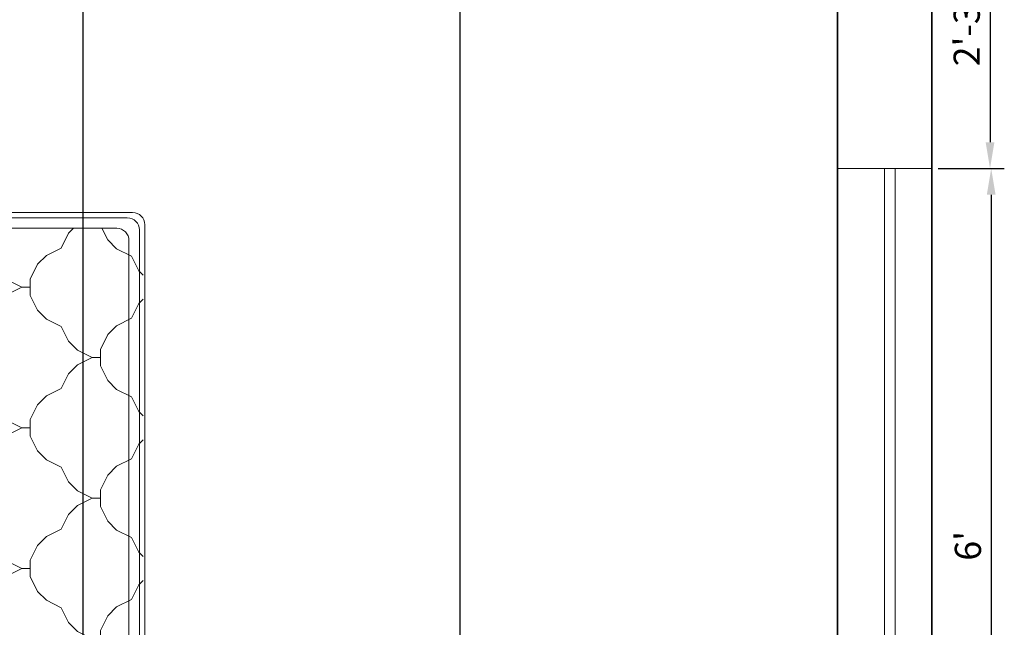
# Model space of a CAD drawing. Units: inches. Extents: x 1624 to 3956, y 1589 to 5028.
# Tile 6 of 16: x 2014 to 2108, y 2133 to 2191. Entities that reach past the tile are written whole.
import ezdxf

# ---------------------------------------------------------------- set-up
doc = ezdxf.new("R2010")
doc.units = ezdxf.units.IN
for name, color, linetype, lineweight in [('A-ANNO-DIMS', 2, 'Continuous', 13), ('A-FURN', 8, 'Continuous', 18), ('A-GLAZ', 4, 'Continuous', 18), ('A-WALL', 7, 'Continuous', 35)]:
    doc.layers.add(name, color=color, linetype=linetype, lineweight=lineweight)
doc.styles.get("Standard").update_dxf_attribs({"font": 'arial.ttf'})
doc.dimstyles.new('Copy of ISO-25', dxfattribs={"dimtxt": 2.5, "dimasz": 2.5, "dimexe": 1.25, "dimexo": 0.625, "dimtad": 1, "dimdec": 1, "dimlunit": 4, "dimtxsty": 'Standard', "dimcen": 2.5, "dimadec": 0, "dimazin": 0, "dimtfac": 1, "dimtdec": 1, "dimtmove": 0, "dimatfit": 3, "dimfxl": 1, "dimarcsym": 0})

# ---------------------------------------------------------------- blocks, each defined once
blk = doc.blocks.new('A$C029D5C69')
for p, q in [((0.4164, 2.0693), (0.4164, 2.0066)), ((2.2315, 2.0693), (0.4164, 2.0693)), ((2.2315, 2.0066), (2.2315, 2.0693)), ((0, 1.606), (0, 2.0066)), ((0, 2.0066), (0.505, 2.0066)), ((0.4164, 2.0066), (2.2315, 2.0066)), ((0.505, 2.0066), (0.505, 1.606)), ((0.5252, 0.0351), (0.5252, 2.0066)), ((0.5403, 0.0502), (0.5403, 2.0066)), ((0.5706, 0.0805), (0.5706, 2.0066)), ((0.6869, 1.966), (0.6666, 2.0066)), ((0.7072, 2.0066), (0.6869, 1.966)), ((1.0902, 1.966), (1.0699, 2.0066)), ((1.1106, 2.0066), (1.0902, 1.966)), ((2.1114, 2.0087), (2.1114, 0.0351)), ((2.6479, 2.0066), (2.1429, 2.0066)), ((2.1429, 2.0066), (2.1429, 1.606)), ((2.6479, 1.606), (2.6479, 2.0066)), ((0.0151, 1.6211), (0.0151, 1.9915)), ((0.0151, 1.9915), (0.4899, 1.9915)), ((0.4899, 1.9915), (0.4899, 1.6211)), ((1.8954, 1.9865), (1.3081, 1.9865)), ((2.6328, 1.9915), (2.158, 1.9915)), ((2.158, 1.9915), (2.158, 1.6211)), ((2.6328, 1.6211), (2.6328, 1.9915)), ((0.2689, 1.9609), (0.2689, 1.6764)), ((0.6869, 1.9425), (0.6869, 1.966)), ((0.6869, 1.9425), (0.6869, 1.966)), ((1.0902, 1.9425), (1.0902, 1.966)), ((1.0902, 1.9425), (1.0902, 1.966)), ((1.8954, 1.9713), (1.3339, 1.9713)), ((1.3849, 1.9713), (1.3656, 1.952)), ((1.3945, 1.9713), (1.3714, 1.9483)), ((1.4249, 1.945), (1.3986, 1.9713)), ((1.4288, 1.9507), (1.4081, 1.9713)), ((1.4476, 1.9507), (1.4288, 1.9507)), ((1.4476, 1.9507), (1.4664, 1.9507)), ((1.487, 1.9713), (1.4664, 1.9507)), ((1.4966, 1.9713), (1.4703, 1.945)), ((1.527, 1.945), (1.5007, 1.9713)), ((1.5309, 1.9507), (1.5102, 1.9713)), ((1.5497, 1.9507), (1.5309, 1.9507)), ((1.5497, 1.9507), (1.5685, 1.9507)), ((1.5891, 1.9713), (1.5685, 1.9507)), ((1.5987, 1.9713), (1.5724, 1.945)), ((1.6291, 1.945), (1.6028, 1.9713)), ((1.633, 1.9507), (1.6123, 1.9713)), ((1.6518, 1.9507), (1.633, 1.9507)), ((1.6518, 1.9507), (1.6706, 1.9507)), ((1.6912, 1.9713), (1.6706, 1.9507)), ((1.7008, 1.9713), (1.6745, 1.945)), ((1.7312, 1.945), (1.7049, 1.9713)), ((1.7351, 1.9507), (1.7144, 1.9713)), ((1.7539, 1.9507), (1.7351, 1.9507)), ((1.7539, 1.9507), (1.7727, 1.9507)), ((1.7933, 1.9713), (1.7727, 1.9507)), ((1.8029, 1.9713), (1.7766, 1.945)), ((1.8333, 1.945), (1.807, 1.9713)), ((1.8372, 1.9507), (1.8165, 1.9713)), ((1.856, 1.9507), (1.8372, 1.9507)), ((1.856, 1.9507), (1.8748, 1.9507)), ((1.8954, 1.9713), (1.8748, 1.9507)), ((1.9043, 1.9707), (1.8787, 1.945)), ((1.9354, 1.945), (1.9114, 1.969)), ((2.379, 1.9609), (2.379, 1.6764)), ((0.6634, 1.9425), (0.621, 1.9213)), ((0.6634, 1.9425), (0.621, 1.9213)), ((0.6869, 1.9425), (0.6634, 1.9425)), ((0.6869, 1.9425), (0.7104, 1.9425)), ((0.7528, 1.9213), (0.7104, 1.9425)), ((0.7528, 1.9213), (0.7104, 1.9425)), ((1.0668, 1.9425), (1.0244, 1.9213)), ((1.0668, 1.9425), (1.0244, 1.9213)), ((1.0902, 1.9425), (1.0668, 1.9425)), ((1.0902, 1.9425), (1.1137, 1.9425)), ((1.1561, 1.9213), (1.1137, 1.9425)), ((1.1561, 1.9213), (1.1137, 1.9425)), ((1.4249, 1.945), (1.4059, 1.926)), ((1.4288, 1.9394), (1.4116, 1.9222)), ((1.4288, 1.9393), (1.4476, 1.9393)), ((1.4664, 1.9393), (1.4476, 1.9393)), ((1.493, 1.9128), (1.4664, 1.9394)), ((1.4986, 1.9167), (1.4703, 1.945)), ((1.527, 1.945), (1.4986, 1.9167)), ((1.5309, 1.9394), (1.5043, 1.9128)), ((1.5309, 1.9393), (1.5497, 1.9393)), ((1.5685, 1.9393), (1.5497, 1.9393)), ((1.595, 1.9128), (1.5685, 1.9394)), ((1.6007, 1.9167), (1.5724, 1.945)), ((1.6291, 1.945), (1.6007, 1.9167)), ((1.633, 1.9394), (1.6064, 1.9128)), ((1.633, 1.9393), (1.6518, 1.9393)), ((1.6706, 1.9393), (1.6518, 1.9393)), ((1.6971, 1.9128), (1.6706, 1.9394)), ((1.7028, 1.9167), (1.6745, 1.945)), ((1.7312, 1.945), (1.7028, 1.9167)), ((1.7351, 1.9394), (1.7085, 1.9128)), ((1.7351, 1.9393), (1.7539, 1.9393)), ((1.7727, 1.9393), (1.7539, 1.9393)), ((1.7992, 1.9128), (1.7727, 1.9394)), ((1.8049, 1.9167), (1.7766, 1.945)), ((1.8333, 1.945), (1.8049, 1.9167)), ((1.8372, 1.9394), (1.8106, 1.9128)), ((1.8372, 1.9393), (1.856, 1.9393)), ((1.8748, 1.9393), (1.856, 1.9393)), ((1.9013, 1.9128), (1.8748, 1.9394)), ((1.907, 1.9167), (1.8787, 1.945)), ((1.9354, 1.945), (1.907, 1.9167)), ((1.9393, 1.9394), (1.9127, 1.9128)), ((1.9393, 1.9393), (1.9404, 1.9393)), ((1.9414, 1.688), (1.9414, 1.931)), ((1.9565, 1.688), (1.9565, 1.931)), ((0.5955, 1.8958), (0.5743, 1.8534)), ((0.621, 1.9213), (0.5955, 1.8958)), ((0.7783, 1.8958), (0.7528, 1.9213)), ((0.7995, 1.8534), (0.7783, 1.8958)), ((0.9989, 1.8958), (0.9777, 1.8534)), ((1.0243, 1.9213), (0.9988, 1.8958)), ((1.1816, 1.8958), (1.1561, 1.9213)), ((1.2028, 1.8534), (1.1816, 1.8958)), ((1.493, 1.8752), (1.493, 1.9128)), ((1.5043, 1.8752), (1.5043, 1.9128)), ((1.595, 1.8752), (1.595, 1.9128)), ((1.6064, 1.8752), (1.6064, 1.9128)), ((1.6971, 1.8752), (1.6971, 1.9128)), ((1.7085, 1.8752), (1.7085, 1.9128)), ((1.7992, 1.8752), (1.7992, 1.9128)), ((1.8106, 1.8752), (1.8106, 1.9128)), ((1.9013, 1.8752), (1.9013, 1.9128)), ((1.9127, 1.8752), (1.9127, 1.9128)), ((1.493, 1.8752), (1.4867, 1.869)), ((1.4986, 1.8713), (1.4922, 1.8648)), ((1.527, 1.8429), (1.4986, 1.8713)), ((1.5309, 1.8486), (1.5043, 1.8752)), ((1.595, 1.8752), (1.5685, 1.8486)), ((1.6007, 1.8713), (1.5724, 1.8429)), ((1.6291, 1.8429), (1.6007, 1.8713)), ((1.633, 1.8486), (1.6064, 1.8752)), ((1.6971, 1.8752), (1.6706, 1.8486)), ((1.7028, 1.8713), (1.6745, 1.8429)), ((1.7312, 1.8429), (1.7028, 1.8713)), ((1.7351, 1.8486), (1.7085, 1.8752)), ((1.7992, 1.8752), (1.7727, 1.8486)), ((1.8049, 1.8713), (1.7766, 1.8429)), ((1.8333, 1.8429), (1.8049, 1.8713)), ((1.8372, 1.8486), (1.8106, 1.8752)), ((1.9013, 1.8752), (1.8748, 1.8486)), ((1.907, 1.8713), (1.8787, 1.8429)), ((1.9354, 1.8429), (1.907, 1.8713)), ((1.9393, 1.8486), (1.9127, 1.8752)), ((0.5743, 1.8534), (0.5706, 1.8515)), ((0.5743, 1.8534), (0.5706, 1.8515)), ((0.8419, 1.8322), (0.7995, 1.8534)), ((0.8419, 1.8322), (0.7995, 1.8534)), ((0.9777, 1.8534), (0.9353, 1.8322)), ((0.9777, 1.8534), (0.9353, 1.8322)), ((1.2452, 1.8322), (1.2028, 1.8534)), ((1.2452, 1.8322), (1.2028, 1.8534)), ((1.527, 1.8429), (1.5242, 1.8401)), ((1.5309, 1.8373), (1.5295, 1.8359)), ((1.5497, 1.8486), (1.5309, 1.8486)), ((1.5309, 1.8373), (1.5497, 1.8373)), ((1.5497, 1.8486), (1.5685, 1.8486)), ((1.5685, 1.8373), (1.5497, 1.8373)), ((1.595, 1.8107), (1.5685, 1.8373)), ((1.6007, 1.8146), (1.5724, 1.8429)), ((1.6291, 1.8429), (1.6007, 1.8146)), ((1.633, 1.8373), (1.6064, 1.8107)), ((1.6518, 1.8486), (1.633, 1.8486)), ((1.633, 1.8373), (1.6518, 1.8373)), ((1.6518, 1.8486), (1.6706, 1.8486)), ((1.6706, 1.8373), (1.6518, 1.8373)), ((1.6971, 1.8107), (1.6706, 1.8373)), ((1.7028, 1.8146), (1.6745, 1.8429)), ((1.7312, 1.8429), (1.7028, 1.8146)), ((1.7351, 1.8373), (1.7085, 1.8107)), ((1.7539, 1.8486), (1.7351, 1.8486)), ((1.7351, 1.8373), (1.7539, 1.8373)), ((1.7539, 1.8486), (1.7727, 1.8486)), ((1.7727, 1.8373), (1.7539, 1.8373)), ((1.7992, 1.8107), (1.7727, 1.8373)), ((1.8049, 1.8146), (1.7766, 1.8429)), ((1.8333, 1.8429), (1.8049, 1.8146)), ((1.8372, 1.8373), (1.8106, 1.8107)), ((1.856, 1.8486), (1.8372, 1.8486)), ((1.8372, 1.8373), (1.856, 1.8373)), ((1.856, 1.8486), (1.8748, 1.8486)), ((1.8748, 1.8373), (1.856, 1.8373)), ((1.9013, 1.8107), (1.8748, 1.8373)), ((1.907, 1.8146), (1.8787, 1.8429)), ((1.9354, 1.8429), (1.907, 1.8146)), ((1.9393, 1.8373), (1.9127, 1.8107)), ((1.9414, 1.8486), (1.9393, 1.8486)), ((1.9393, 1.8373), (1.9414, 1.8373)), ((0.1267, 1.8186), (0.4111, 1.8186)), ((0.8674, 1.8067), (0.8419, 1.8322)), ((0.9352, 1.8322), (0.9097, 1.8067)), ((1.2707, 1.8067), (1.2452, 1.8322)), ((1.595, 1.7806), (1.595, 1.8107)), ((1.6064, 1.7731), (1.6064, 1.8107)), ((1.6971, 1.7731), (1.6971, 1.8107)), ((1.7085, 1.7731), (1.7085, 1.8107)), ((1.7992, 1.7731), (1.7992, 1.8107)), ((1.8106, 1.7731), (1.8106, 1.8107)), ((1.9013, 1.7731), (1.9013, 1.8107)), ((1.9127, 1.7731), (1.9127, 1.8107)), ((2.2367, 1.8186), (2.5212, 1.8186)), ((0.8886, 1.7643), (0.8674, 1.8067)), ((0.9098, 1.8067), (0.8886, 1.7643)), ((1.2919, 1.7643), (1.2707, 1.8067)), ((0.8886, 1.7408), (0.8886, 1.7643)), ((1.2981, 1.7768), (1.2919, 1.7643)), ((1.2919, 1.7519), (1.2919, 1.7643)), ((1.633, 1.7465), (1.6064, 1.7731)), ((1.6971, 1.7731), (1.6706, 1.7465)), ((1.7028, 1.7692), (1.6745, 1.7408)), ((1.7312, 1.7408), (1.7028, 1.7692)), ((1.7351, 1.7465), (1.7085, 1.7731)), ((1.7992, 1.7731), (1.7727, 1.7465)), ((1.8049, 1.7692), (1.7766, 1.7408)), ((1.8333, 1.7408), (1.8049, 1.7692)), ((1.8372, 1.7465), (1.8106, 1.7731)), ((1.9013, 1.7731), (1.8748, 1.7465)), ((1.907, 1.7692), (1.8787, 1.7408)), ((1.9354, 1.7408), (1.907, 1.7692)), ((1.9393, 1.7465), (1.9127, 1.7731)), ((0.8651, 1.7408), (0.8227, 1.7196)), ((0.8651, 1.7408), (0.8227, 1.7196)), ((0.912, 1.7408), (0.8651, 1.7408)), ((0.9544, 1.7196), (0.912, 1.7408)), ((0.9544, 1.7196), (0.912, 1.7408)), ((1.2684, 1.7408), (1.226, 1.7196)), ((1.2684, 1.7408), (1.226, 1.7196)), ((1.2885, 1.7408), (1.2684, 1.7408)), ((1.6518, 1.7465), (1.633, 1.7465)), ((1.6443, 1.7352), (1.6518, 1.7352)), ((1.6518, 1.7465), (1.6706, 1.7465)), ((1.6706, 1.7352), (1.6518, 1.7352)), ((1.6971, 1.7086), (1.6706, 1.7352)), ((1.7028, 1.7125), (1.6745, 1.7408)), ((1.7312, 1.7408), (1.7028, 1.7125)), ((1.7351, 1.7352), (1.7085, 1.7086)), ((1.7539, 1.7465), (1.7351, 1.7465)), ((1.7351, 1.7352), (1.7539, 1.7352)), ((1.7539, 1.7465), (1.7727, 1.7465)), ((1.7727, 1.7352), (1.7539, 1.7352)), ((1.7992, 1.7086), (1.7727, 1.7352)), ((1.8049, 1.7125), (1.7766, 1.7408)), ((1.8333, 1.7408), (1.8049, 1.7125)), ((1.8372, 1.7352), (1.8106, 1.7086)), ((1.856, 1.7465), (1.8372, 1.7465)), ((1.8372, 1.7352), (1.856, 1.7352)), ((1.856, 1.7465), (1.8748, 1.7465)), ((1.8748, 1.7352), (1.856, 1.7352)), ((1.9013, 1.7086), (1.8748, 1.7352)), ((1.907, 1.7125), (1.8787, 1.7408)), ((1.9354, 1.7408), (1.907, 1.7125)), ((1.9393, 1.7352), (1.9127, 1.7086)), ((1.9414, 1.7465), (1.9393, 1.7465)), ((1.9393, 1.7352), (1.9414, 1.7352)), ((0.5766, 1.6941), (0.5706, 1.7002)), ((0.8227, 1.7196), (0.7972, 1.6941)), ((0.98, 1.6941), (0.9545, 1.7196)), ((1.226, 1.7196), (1.2005, 1.6941)), ((1.6971, 1.682), (1.6971, 1.7086)), ((1.7085, 1.671), (1.7085, 1.7086)), ((1.7992, 1.671), (1.7992, 1.7086)), ((1.8106, 1.671), (1.8106, 1.7086)), ((1.9013, 1.671), (1.9013, 1.7086)), ((1.9127, 1.671), (1.9127, 1.7086)), ((2.5551, 1.6275), (2.5551, 1.696)), ((0.5978, 1.6517), (0.5766, 1.6941)), ((0.7972, 1.6941), (0.776, 1.6517)), ((1.0011, 1.6517), (0.9799, 1.6941)), ((1.2005, 1.6941), (1.1793, 1.6517)), ((1.7318, 1.6477), (1.7085, 1.671)), ((1.7992, 1.671), (1.7759, 1.6477)), ((1.8339, 1.6477), (1.8106, 1.671)), ((1.9013, 1.671), (1.878, 1.6477)), ((1.926, 1.6577), (1.9127, 1.671)), ((0.6402, 1.6305), (0.5978, 1.6517)), ((0.6402, 1.6305), (0.5978, 1.6517)), ((0.776, 1.6517), (0.7336, 1.6305)), ((0.776, 1.6517), (0.7336, 1.6305)), ((1.0435, 1.6305), (1.0011, 1.6517)), ((1.0435, 1.6305), (1.0011, 1.6517)), ((1.1793, 1.6517), (1.1369, 1.6305)), ((1.1793, 1.6517), (1.1369, 1.6305)), ((1.8961, 1.6477), (1.7289, 1.6477)), ((1.8049, 1.6671), (1.7855, 1.6477)), ((1.8244, 1.6477), (1.8049, 1.6671)), ((1.907, 1.6671), (1.8876, 1.6477)), ((1.9202, 1.6539), (1.907, 1.6671)), ((0.4899, 1.6211), (0.0151, 1.6211)), ((0.6657, 1.605), (0.6402, 1.6305)), ((0.7336, 1.6305), (0.7081, 1.605)), ((1.0691, 1.605), (1.0436, 1.6305)), ((1.1369, 1.6305), (1.1114, 1.605)), ((1.8961, 1.6325), (1.7422, 1.6325)), ((2.158, 1.6211), (2.6328, 1.6211)), ((0.505, 1.606), (0, 1.606)), ((0.6869, 1.5626), (0.6657, 1.605)), ((0.7081, 1.605), (0.6869, 1.5626)), ((1.0902, 1.5626), (1.069, 1.605)), ((1.1114, 1.605), (1.0902, 1.5626)), ((2.1429, 1.606), (2.6479, 1.606)), ((0.6869, 1.5392), (0.6869, 1.5626)), ((0.6869, 1.5392), (0.6869, 1.5626)), ((1.0902, 1.5392), (1.0902, 1.5626)), ((1.0902, 1.5392), (1.0902, 1.5626)), ((0.6634, 1.5391), (0.621, 1.5179)), ((0.6634, 1.5391), (0.621, 1.5179)), ((0.6869, 1.5392), (0.6634, 1.5392)), ((0.6869, 1.5392), (0.7104, 1.5392)), ((0.7528, 1.5179), (0.7104, 1.5391)), ((0.7528, 1.5179), (0.7104, 1.5391)), ((1.0668, 1.5391), (1.0244, 1.5179)), ((1.0668, 1.5391), (1.0244, 1.5179)), ((1.0902, 1.5392), (1.0668, 1.5392)), ((1.0902, 1.5392), (1.1137, 1.5392)), ((1.1561, 1.5179), (1.1137, 1.5391)), ((1.1561, 1.5179), (1.1137, 1.5391)), ((1.4534, 1.5308), (1.4277, 1.5179)), ((1.4534, 1.5308), (1.4277, 1.5179)), ((0.621, 1.5179), (0.5955, 1.4924)), ((0.7783, 1.4924), (0.7528, 1.5179)), ((1.0243, 1.5179), (0.9988, 1.4924)), ((1.1816, 1.4924), (1.1561, 1.5179)), ((1.4277, 1.5179), (1.4022, 1.4924)), ((0.5955, 1.4925), (0.5743, 1.4501)), ((0.7995, 1.4501), (0.7783, 1.4925)), ((0.9989, 1.4925), (0.9777, 1.4501)), ((1.2028, 1.4501), (1.1816, 1.4925)), ((1.4022, 1.4925), (1.381, 1.4501)), ((0.5743, 1.45), (0.5706, 1.4481)), ((0.5743, 1.45), (0.5706, 1.4481)), ((0.8419, 1.4288), (0.7995, 1.45)), ((0.8419, 1.4288), (0.7995, 1.45)), ((0.9777, 1.45), (0.9353, 1.4288)), ((0.9777, 1.45), (0.9353, 1.4288)), ((1.2452, 1.4288), (1.2028, 1.45)), ((1.2452, 1.4288), (1.2028, 1.45)), ((1.381, 1.45), (1.3386, 1.4288)), ((1.381, 1.45), (1.3386, 1.4288)), ((1.6062, 1.4501), (1.5966, 1.4692)), ((1.6486, 1.4288), (1.6062, 1.45)), ((1.6486, 1.4288), (1.6062, 1.45)), ((0.8674, 1.4033), (0.8419, 1.4288)), ((0.9352, 1.4288), (0.9097, 1.4033)), ((1.2707, 1.4033), (1.2452, 1.4288)), ((1.3386, 1.4288), (1.3131, 1.4033)), ((1.6741, 1.4033), (1.6486, 1.4288)), ((0.5403, 1.4117), (0.5706, 1.4117)), ((0.8886, 1.361), (0.8674, 1.4034)), ((0.9098, 1.4034), (0.8886, 1.361)), ((1.2919, 1.361), (1.2707, 1.4034)), ((1.3131, 1.4034), (1.2919, 1.361)), ((1.6953, 1.361), (1.6741, 1.4034)), ((1.714, 1.3984), (1.6953, 1.361)), ((0.8886, 1.3375), (0.8886, 1.3609)), ((1.2919, 1.3375), (1.2919, 1.3609)), ((1.6953, 1.3375), (1.6953, 1.3609)), ((0.8651, 1.3374), (0.8227, 1.3162)), ((0.8651, 1.3374), (0.8227, 1.3162)), ((0.912, 1.3375), (0.8651, 1.3375)), ((0.9544, 1.3162), (0.912, 1.3374)), ((0.9544, 1.3162), (0.912, 1.3374)), ((1.2684, 1.3374), (1.226, 1.3162)), ((1.2684, 1.3374), (1.226, 1.3162)), ((1.3154, 1.3375), (1.2684, 1.3375)), ((1.3578, 1.3162), (1.3154, 1.3374)), ((1.3578, 1.3162), (1.3154, 1.3374)), ((1.6718, 1.3374), (1.6294, 1.3162)), ((1.6718, 1.3374), (1.6294, 1.3162)), ((1.7187, 1.3375), (1.6718, 1.3375)), ((1.7611, 1.3162), (1.7187, 1.3374)), ((1.7611, 1.3162), (1.7187, 1.3374)), ((0.8227, 1.3163), (0.7972, 1.2908)), ((0.98, 1.2908), (0.9545, 1.3163)), ((1.226, 1.3163), (1.2005, 1.2908)), ((1.3833, 1.2908), (1.3578, 1.3163)), ((1.6294, 1.3163), (1.6039, 1.2908)), ((1.7867, 1.2908), (1.7611, 1.3163)), ((0.5766, 1.2908), (0.5706, 1.2968)), ((0.5978, 1.2484), (0.5766, 1.2908)), ((0.7972, 1.2908), (0.776, 1.2484)), ((1.0011, 1.2484), (0.9799, 1.2908)), ((1.2005, 1.2908), (1.1793, 1.2484)), ((1.4045, 1.2484), (1.3833, 1.2908)), ((1.6039, 1.2908), (1.5827, 1.2484)), ((1.8078, 1.2484), (1.7866, 1.2908)), ((0.6402, 1.2271), (0.5978, 1.2483)), ((0.6402, 1.2271), (0.5978, 1.2483)), ((0.776, 1.2483), (0.7336, 1.2271)), ((0.776, 1.2483), (0.7336, 1.2271)), ((1.0435, 1.2271), (1.0011, 1.2483)), ((1.0435, 1.2271), (1.0011, 1.2483)), ((1.1793, 1.2483), (1.1369, 1.2271)), ((1.1793, 1.2483), (1.1369, 1.2271)), ((1.4469, 1.2271), (1.4045, 1.2483)), ((1.4469, 1.2271), (1.4045, 1.2483)), ((1.5827, 1.2483), (1.5403, 1.2271)), ((1.5827, 1.2483), (1.5403, 1.2271)), ((1.8502, 1.2271), (1.8078, 1.2483)), ((1.8502, 1.2271), (1.8078, 1.2483)), ((0.6657, 1.2017), (0.6402, 1.2272)), ((0.7336, 1.2272), (0.7081, 1.2017)), ((1.0691, 1.2017), (1.0436, 1.2272)), ((1.1369, 1.2272), (1.1114, 1.2017)), ((1.4724, 1.2017), (1.4469, 1.2272)), ((1.5403, 1.2272), (1.5148, 1.2017)), ((1.8758, 1.2017), (1.8503, 1.2272)), ((0.5403, 1.21), (0.5706, 1.21)), ((0.6869, 1.1593), (0.6657, 1.2017)), ((0.7081, 1.2017), (0.6869, 1.1593)), ((1.0902, 1.1593), (1.069, 1.2017)), ((1.1114, 1.2017), (1.0902, 1.1593)), ((1.4936, 1.1593), (1.4724, 1.2017)), ((1.5148, 1.2017), (1.4936, 1.1593)), ((1.8969, 1.1593), (1.8757, 1.2017)), ((1.9181, 1.2017), (1.8969, 1.1593)), ((1.9215, 1.2051), (1.9181, 1.2017)), ((0.6869, 1.1358), (0.6869, 1.1593)), ((0.6869, 1.1358), (0.6869, 1.1593)), ((1.0902, 1.1358), (1.0902, 1.1593)), ((1.0902, 1.1358), (1.0902, 1.1593)), ((1.4936, 1.1358), (1.4936, 1.1593)), ((1.4936, 1.1358), (1.4936, 1.1593)), ((1.8969, 1.1358), (1.8969, 1.1593)), ((1.8969, 1.1358), (1.8969, 1.1593)), ((0.6634, 1.1358), (0.621, 1.1146)), ((0.6634, 1.1358), (0.621, 1.1146)), ((0.6869, 1.1358), (0.6634, 1.1358)), ((0.6869, 1.1358), (0.7104, 1.1358)), ((0.7528, 1.1146), (0.7104, 1.1358)), ((0.7528, 1.1146), (0.7104, 1.1358)), ((1.0668, 1.1358), (1.0244, 1.1146)), ((1.0668, 1.1358), (1.0244, 1.1146)), ((1.0902, 1.1358), (1.0668, 1.1358)), ((1.0902, 1.1358), (1.1137, 1.1358)), ((1.1561, 1.1146), (1.1137, 1.1358)), ((1.1561, 1.1146), (1.1137, 1.1358)), ((1.4701, 1.1358), (1.4277, 1.1146)), ((1.4701, 1.1358), (1.4277, 1.1146)), ((1.4936, 1.1358), (1.4701, 1.1358)), ((1.4936, 1.1358), (1.5171, 1.1358)), ((1.5595, 1.1146), (1.5171, 1.1358)), ((1.5595, 1.1146), (1.5171, 1.1358)), ((1.8735, 1.1358), (1.8311, 1.1146)), ((1.8735, 1.1358), (1.8311, 1.1146)), ((1.8969, 1.1358), (1.8735, 1.1358)), ((1.8969, 1.1358), (1.9204, 1.1358)), ((1.9628, 1.1146), (1.9204, 1.1358)), ((1.9628, 1.1146), (1.9204, 1.1358)), ((0.621, 1.1146), (0.5955, 1.0891)), ((0.7783, 1.0891), (0.7528, 1.1146)), ((1.0243, 1.1146), (0.9988, 1.0891)), ((1.1816, 1.0891), (1.1561, 1.1146)), ((1.4277, 1.1146), (1.4022, 1.0891)), ((1.585, 1.0891), (1.5595, 1.1146)), ((1.831, 1.1146), (1.8055, 1.0891)), ((1.9883, 1.0891), (1.9628, 1.1146)), ((0.5955, 1.0891), (0.5743, 1.0467)), ((0.7995, 1.0467), (0.7783, 1.0891)), ((0.9989, 1.0891), (0.9777, 1.0467)), ((1.2028, 1.0467), (1.1816, 1.0891)), ((1.4022, 1.0891), (1.381, 1.0467)), ((1.6062, 1.0467), (1.585, 1.0891)), ((1.8056, 1.0891), (1.7844, 1.0467)), ((2.0095, 1.0467), (1.9883, 1.0891)), ((0.5743, 1.0467), (0.5706, 1.0448)), ((0.5743, 1.0467), (0.5706, 1.0448)), ((0.8419, 1.0255), (0.7995, 1.0467)), ((0.8419, 1.0255), (0.7995, 1.0467)), ((0.9777, 1.0467), (0.9353, 1.0255)), ((0.9777, 1.0467), (0.9353, 1.0255)), ((1.2452, 1.0255), (1.2028, 1.0467)), ((1.2452, 1.0255), (1.2028, 1.0467)), ((1.381, 1.0467), (1.3386, 1.0255)), ((1.381, 1.0467), (1.3386, 1.0255)), ((1.6486, 1.0255), (1.6062, 1.0467)), ((1.6486, 1.0255), (1.6062, 1.0467)), ((1.7844, 1.0467), (1.742, 1.0255)), ((1.7844, 1.0467), (1.742, 1.0255)), ((2.0276, 1.0376), (2.0095, 1.0467)), ((2.0276, 1.0376), (2.0095, 1.0467)), ((0.8674, 1), (0.8419, 1.0255)), ((0.9352, 1.0255), (0.9097, 1)), ((1.2707, 1), (1.2452, 1.0255)), ((1.3386, 1.0255), (1.3131, 1)), ((1.6741, 1), (1.6486, 1.0255)), ((1.7419, 1.0255), (1.7164, 1)), ((0.8886, 0.9576), (0.8674, 1)), ((0.9098, 1), (0.8886, 0.9576)), ((1.2919, 0.9576), (1.2707, 1)), ((1.3131, 1), (1.2919, 0.9576)), ((1.6953, 0.9576), (1.6741, 1)), ((1.7165, 1), (1.6953, 0.9576)), ((0.8651, 0.9341), (0.8227, 0.9129)), ((0.8651, 0.9341), (0.8227, 0.9129)), ((0.912, 0.9341), (0.8651, 0.9341)), ((0.8886, 0.9341), (0.8886, 0.9576)), ((0.9544, 0.9129), (0.912, 0.9341)), ((0.9544, 0.9129), (0.912, 0.9341)), ((1.2684, 0.9341), (1.226, 0.9129)), ((1.2684, 0.9341), (1.226, 0.9129)), ((1.3154, 0.9341), (1.2684, 0.9341)), ((1.2919, 0.9341), (1.2919, 0.9576)), ((1.3578, 0.9129), (1.3154, 0.9341)), ((1.3578, 0.9129), (1.3154, 0.9341)), ((1.6718, 0.9341), (1.6294, 0.9129)), ((1.6718, 0.9341), (1.6294, 0.9129)), ((1.7187, 0.9341), (1.6718, 0.9341)), ((1.6953, 0.9341), (1.6953, 0.9576)), ((1.7611, 0.9129), (1.7187, 0.9341)), ((1.7611, 0.9129), (1.7187, 0.9341)), ((2.066, 0.9457), (2.066, 0.0805)), ((0.8227, 0.9129), (0.7972, 0.8874)), ((0.98, 0.8874), (0.9545, 0.9129)), ((1.226, 0.9129), (1.2005, 0.8874)), ((1.3833, 0.8874), (1.3578, 0.9129)), ((1.6294, 0.9129), (1.6039, 0.8874)), ((1.7867, 0.8874), (1.7611, 0.9129)), ((2.0327, 0.9129), (2.0072, 0.8874)), ((2.066, 0.9295), (2.0327, 0.9129)), ((2.066, 0.9295), (2.0327, 0.9129)), ((0.5766, 0.8874), (0.5706, 0.8935)), ((0.5978, 0.845), (0.5766, 0.8874)), ((0.7972, 0.8874), (0.776, 0.845)), ((1.0011, 0.845), (0.9799, 0.8874)), ((1.2005, 0.8874), (1.1793, 0.845)), ((1.4045, 0.845), (1.3833, 0.8874)), ((1.6039, 0.8874), (1.5827, 0.845)), ((1.8078, 0.845), (1.7866, 0.8874)), ((2.0072, 0.8874), (1.986, 0.845)), ((0.6402, 0.8238), (0.5978, 0.845)), ((0.6402, 0.8238), (0.5978, 0.845)), ((0.6657, 0.7983), (0.6402, 0.8238)), ((0.7336, 0.8238), (0.7081, 0.7983)), ((0.776, 0.845), (0.7336, 0.8238)), ((0.776, 0.845), (0.7336, 0.8238)), ((1.0435, 0.8238), (1.0011, 0.845)), ((1.0435, 0.8238), (1.0011, 0.845)), ((1.0691, 0.7983), (1.0436, 0.8238)), ((1.1369, 0.8238), (1.1114, 0.7983)), ((1.1793, 0.845), (1.1369, 0.8238)), ((1.1793, 0.845), (1.1369, 0.8238)), ((1.4469, 0.8238), (1.4045, 0.845)), ((1.4469, 0.8238), (1.4045, 0.845)), ((1.4724, 0.7983), (1.4469, 0.8238)), ((1.5403, 0.8238), (1.5148, 0.7983)), ((1.5827, 0.845), (1.5403, 0.8238)), ((1.5827, 0.845), (1.5403, 0.8238)), ((1.8502, 0.8238), (1.8078, 0.845)), ((1.8502, 0.8238), (1.8078, 0.845)), ((1.8758, 0.7983), (1.8503, 0.8238)), ((1.9436, 0.8238), (1.9181, 0.7983)), ((1.986, 0.845), (1.9436, 0.8238)), ((1.986, 0.845), (1.9436, 0.8238)), ((2.0962, 0.8369), (2.0962, 0.0502)), ((0.6869, 0.7559), (0.6657, 0.7983)), ((0.7081, 0.7983), (0.6869, 0.7559)), ((1.0902, 0.7559), (1.069, 0.7983)), ((1.1114, 0.7983), (1.0902, 0.7559)), ((1.4936, 0.7559), (1.4724, 0.7983)), ((1.5148, 0.7983), (1.4936, 0.7559)), ((1.8969, 0.7559), (1.8757, 0.7983)), ((1.9181, 0.7983), (1.8969, 0.7559)), ((0.6869, 0.7325), (0.6869, 0.7559)), ((0.6869, 0.7325), (0.6869, 0.7559)), ((1.0902, 0.7325), (1.0902, 0.7559)), ((1.0902, 0.7325), (1.0902, 0.7559)), ((1.2024, 0.7028), (1.2503, 0.7507)), ((1.4936, 0.7325), (1.4936, 0.7559)), ((1.4936, 0.7325), (1.4936, 0.7559)), ((1.8969, 0.7325), (1.8969, 0.7559)), ((1.8969, 0.7325), (1.8969, 0.7559)), ((0.621, 0.7113), (0.5955, 0.6858)), ((0.6634, 0.7324), (0.621, 0.7112)), ((0.6634, 0.7324), (0.621, 0.7112)), ((0.6869, 0.7325), (0.6634, 0.7325)), ((0.6869, 0.7325), (0.7104, 0.7325)), ((0.7528, 0.7112), (0.7104, 0.7324)), ((0.7528, 0.7112), (0.7104, 0.7324)), ((0.7783, 0.6858), (0.7528, 0.7113)), ((1.0243, 0.7113), (0.9988, 0.6858)), ((1.0668, 0.7324), (1.0244, 0.7112)), ((1.0668, 0.7324), (1.0244, 0.7112)), ((1.0902, 0.7325), (1.0668, 0.7325)), ((1.0902, 0.7325), (1.1137, 0.7325)), ((1.1561, 0.7112), (1.1137, 0.7324)), ((1.1561, 0.7112), (1.1137, 0.7324)), ((1.1816, 0.6858), (1.1561, 0.7113)), ((1.4277, 0.7113), (1.4022, 0.6858)), ((1.4701, 0.7324), (1.4277, 0.7112)), ((1.4701, 0.7324), (1.4277, 0.7112)), ((1.4936, 0.7325), (1.4701, 0.7325)), ((1.4936, 0.7325), (1.5171, 0.7325)), ((1.5595, 0.7112), (1.5171, 0.7324)), ((1.5595, 0.7112), (1.5171, 0.7324)), ((1.585, 0.6858), (1.5595, 0.7113)), ((1.831, 0.7113), (1.8055, 0.6858)), ((1.8735, 0.7324), (1.8311, 0.7112)), ((1.8735, 0.7324), (1.8311, 0.7112)), ((1.8969, 0.7325), (1.8735, 0.7325)), ((1.8969, 0.7325), (1.9204, 0.7325)), ((1.9628, 0.7112), (1.9204, 0.7324)), ((1.9628, 0.7112), (1.9204, 0.7324)), ((1.9883, 0.6858), (1.9628, 0.7113)), ((0.5955, 0.6858), (0.5743, 0.6434)), ((0.7995, 0.6434), (0.7783, 0.6858)), ((0.9989, 0.6858), (0.9777, 0.6434)), ((1.2028, 0.6434), (1.1816, 0.6858)), ((1.4022, 0.6858), (1.381, 0.6434)), ((1.6062, 0.6434), (1.585, 0.6858)), ((1.8056, 0.6858), (1.7844, 0.6434)), ((2.0095, 0.6434), (1.9883, 0.6858)), ((0.5743, 0.6433), (0.5706, 0.6414)), ((0.5743, 0.6433), (0.5706, 0.6414)), ((0.8419, 0.6221), (0.7995, 0.6433)), ((0.8419, 0.6221), (0.7995, 0.6433)), ((0.8674, 0.5967), (0.8419, 0.6222)), ((0.9352, 0.6222), (0.9097, 0.5967)), ((0.9777, 0.6433), (0.9353, 0.6221)), ((0.9777, 0.6433), (0.9353, 0.6221)), ((1.2452, 0.6221), (1.2028, 0.6433)), ((1.2452, 0.6221), (1.2028, 0.6433)), ((1.2707, 0.5967), (1.2452, 0.6222)), ((1.3386, 0.6222), (1.3131, 0.5967)), ((1.381, 0.6433), (1.3386, 0.6221)), ((1.381, 0.6433), (1.3386, 0.6221)), ((1.6486, 0.6221), (1.6062, 0.6433)), ((1.6486, 0.6221), (1.6062, 0.6433)), ((1.6741, 0.5967), (1.6486, 0.6222)), ((1.7419, 0.6222), (1.7164, 0.5967)), ((1.7844, 0.6433), (1.742, 0.6221)), ((1.7844, 0.6433), (1.742, 0.6221)), ((2.0519, 0.6221), (2.0095, 0.6433)), ((2.0519, 0.6221), (2.0095, 0.6433)), ((2.066, 0.6081), (2.0519, 0.6222)), ((0.8886, 0.5543), (0.8674, 0.5967)), ((0.9098, 0.5967), (0.8886, 0.5543)), ((1.2919, 0.5543), (1.2707, 0.5967)), ((1.3131, 0.5967), (1.2919, 0.5543)), ((1.6953, 0.5543), (1.6741, 0.5967)), ((1.7165, 0.5967), (1.6953, 0.5543)), ((0.8886, 0.5308), (0.8886, 0.5543)), ((1.2919, 0.5308), (1.2919, 0.5543)), ((1.6953, 0.5308), (1.6953, 0.5543)), ((0.8227, 0.5096), (0.7972, 0.4841)), ((0.8651, 0.5308), (0.8227, 0.5096)), ((0.8651, 0.5308), (0.8227, 0.5096)), ((0.912, 0.5308), (0.8651, 0.5308)), ((0.9544, 0.5096), (0.912, 0.5308)), ((0.9544, 0.5096), (0.912, 0.5308)), ((0.98, 0.4841), (0.9545, 0.5096)), ((1.226, 0.5096), (1.2005, 0.4841)), ((1.2684, 0.5308), (1.226, 0.5096)), ((1.2684, 0.5308), (1.226, 0.5096)), ((1.3154, 0.5308), (1.2684, 0.5308)), ((1.3578, 0.5096), (1.3154, 0.5308)), ((1.3578, 0.5096), (1.3154, 0.5308)), ((1.3833, 0.4841), (1.3578, 0.5096)), ((1.6294, 0.5096), (1.6039, 0.4841)), ((1.6718, 0.5308), (1.6294, 0.5096)), ((1.6718, 0.5308), (1.6294, 0.5096)), ((1.7187, 0.5308), (1.6718, 0.5308)), ((1.7611, 0.5096), (1.7187, 0.5308)), ((1.7611, 0.5096), (1.7187, 0.5308)), ((1.7867, 0.4841), (1.7611, 0.5096)), ((2.0327, 0.5096), (2.0072, 0.4841)), ((2.066, 0.5262), (2.0327, 0.5096)), ((2.066, 0.5262), (2.0327, 0.5096)), ((0.5766, 0.4841), (0.5706, 0.4901)), ((0.5978, 0.4417), (0.5766, 0.4841)), ((0.7972, 0.4841), (0.776, 0.4417)), ((1.0011, 0.4417), (0.9799, 0.4841)), ((1.2005, 0.4841), (1.1793, 0.4417)), ((1.4045, 0.4417), (1.3833, 0.4841)), ((1.6039, 0.4841), (1.5827, 0.4417)), ((1.8078, 0.4417), (1.7866, 0.4841)), ((2.0072, 0.4841), (1.986, 0.4417)), ((0.6402, 0.4205), (0.5978, 0.4417)), ((0.6402, 0.4205), (0.5978, 0.4417)), ((0.776, 0.4417), (0.7336, 0.4205)), ((0.776, 0.4417), (0.7336, 0.4205)), ((1.0435, 0.4205), (1.0011, 0.4417)), ((1.0435, 0.4205), (1.0011, 0.4417)), ((1.1793, 0.4417), (1.1369, 0.4205)), ((1.1793, 0.4417), (1.1369, 0.4205)), ((1.4469, 0.4205), (1.4045, 0.4417)), ((1.4469, 0.4205), (1.4045, 0.4417)), ((1.5827, 0.4417), (1.5403, 0.4205)), ((1.5827, 0.4417), (1.5403, 0.4205)), ((1.8502, 0.4205), (1.8078, 0.4417)), ((1.8502, 0.4205), (1.8078, 0.4417)), ((1.986, 0.4417), (1.9436, 0.4205)), ((1.986, 0.4417), (1.9436, 0.4205)), ((0.6657, 0.395), (0.6402, 0.4205)), ((0.7336, 0.4205), (0.7081, 0.395)), ((1.0691, 0.395), (1.0436, 0.4205)), ((1.1369, 0.4205), (1.1114, 0.395)), ((1.4724, 0.395), (1.4469, 0.4205)), ((1.5403, 0.4205), (1.5148, 0.395)), ((1.8758, 0.395), (1.8503, 0.4205)), ((1.9436, 0.4205), (1.9181, 0.395)), ((0.6869, 0.3526), (0.6657, 0.395)), ((0.7081, 0.395), (0.6869, 0.3526)), ((1.0902, 0.3526), (1.069, 0.395)), ((1.1114, 0.395), (1.0902, 0.3526)), ((1.4936, 0.3526), (1.4724, 0.395)), ((1.5148, 0.395), (1.4936, 0.3526)), ((1.8969, 0.3526), (1.8757, 0.395)), ((1.9181, 0.395), (1.8969, 0.3526)), ((0.6869, 0.3291), (0.6869, 0.3526)), ((0.6869, 0.3291), (0.6869, 0.3526)), ((1.0902, 0.3291), (1.0902, 0.3526)), ((1.0902, 0.3291), (1.0902, 0.3526)), ((1.4936, 0.3291), (1.4936, 0.3526)), ((1.4936, 0.3291), (1.4936, 0.3526)), ((1.8969, 0.3291), (1.8969, 0.3526)), ((1.8969, 0.3291), (1.8969, 0.3526)), ((0.6634, 0.3291), (0.621, 0.3079)), ((0.6634, 0.3291), (0.621, 0.3079)), ((0.6869, 0.3291), (0.6634, 0.3291)), ((0.6869, 0.3291), (0.7104, 0.3291)), ((0.7528, 0.3079), (0.7104, 0.3291)), ((0.7528, 0.3079), (0.7104, 0.3291)), ((1.0668, 0.3291), (1.0244, 0.3079)), ((1.0668, 0.3291), (1.0244, 0.3079)), ((1.0902, 0.3291), (1.0668, 0.3291)), ((1.0902, 0.3291), (1.1137, 0.3291)), ((1.1561, 0.3079), (1.1137, 0.3291)), ((1.1561, 0.3079), (1.1137, 0.3291)), ((1.4701, 0.3291), (1.4277, 0.3079)), ((1.4701, 0.3291), (1.4277, 0.3079)), ((1.4936, 0.3291), (1.4701, 0.3291)), ((1.4936, 0.3291), (1.5171, 0.3291)), ((1.5595, 0.3079), (1.5171, 0.3291)), ((1.5595, 0.3079), (1.5171, 0.3291)), ((1.8735, 0.3291), (1.8311, 0.3079)), ((1.8735, 0.3291), (1.8311, 0.3079)), ((1.8969, 0.3291), (1.8735, 0.3291)), ((1.8969, 0.3291), (1.9204, 0.3291)), ((1.9628, 0.3079), (1.9204, 0.3291)), ((1.9628, 0.3079), (1.9204, 0.3291)), ((0.621, 0.3079), (0.5955, 0.2824)), ((0.7783, 0.2824), (0.7528, 0.3079)), ((1.0243, 0.3079), (0.9988, 0.2824)), ((1.1816, 0.2824), (1.1561, 0.3079)), ((1.4277, 0.3079), (1.4022, 0.2824)), ((1.585, 0.2824), (1.5595, 0.3079)), ((1.831, 0.3079), (1.8055, 0.2824)), ((1.9883, 0.2824), (1.9628, 0.3079)), ((0.5955, 0.2824), (0.5743, 0.24)), ((0.7995, 0.24), (0.7783, 0.2824)), ((0.9989, 0.2824), (0.9777, 0.24)), ((1.2028, 0.24), (1.1816, 0.2824)), ((1.4022, 0.2824), (1.381, 0.24)), ((1.6062, 0.24), (1.585, 0.2824)), ((1.8056, 0.2824), (1.7844, 0.24)), ((2.0095, 0.24), (1.9883, 0.2824)), ((0.5743, 0.24), (0.5706, 0.2381)), ((0.5743, 0.24), (0.5706, 0.2381)), ((0.8419, 0.2188), (0.7995, 0.24)), ((0.8419, 0.2188), (0.7995, 0.24)), ((0.9777, 0.24), (0.9353, 0.2188)), ((0.9777, 0.24), (0.9353, 0.2188)), ((1.2452, 0.2188), (1.2028, 0.24)), ((1.2452, 0.2188), (1.2028, 0.24)), ((1.381, 0.24), (1.3386, 0.2188)), ((1.381, 0.24), (1.3386, 0.2188)), ((1.6486, 0.2188), (1.6062, 0.24)), ((1.6486, 0.2188), (1.6062, 0.24)), ((1.7844, 0.24), (1.742, 0.2188)), ((1.7844, 0.24), (1.742, 0.2188)), ((2.0519, 0.2188), (2.0095, 0.24)), ((2.0519, 0.2188), (2.0095, 0.24)), ((0.8674, 0.1933), (0.8419, 0.2188)), ((0.9352, 0.2188), (0.9097, 0.1933)), ((1.2707, 0.1933), (1.2452, 0.2188)), ((1.3386, 0.2188), (1.3131, 0.1933)), ((1.6741, 0.1933), (1.6486, 0.2188)), ((1.7419, 0.2188), (1.7164, 0.1933)), ((2.066, 0.2047), (2.0519, 0.2188)), ((0.8886, 0.1509), (0.8674, 0.1933)), ((0.9098, 0.1933), (0.8886, 0.1509)), ((1.2919, 0.1509), (1.2707, 0.1933)), ((1.3131, 0.1933), (1.2919, 0.1509)), ((1.6953, 0.1509), (1.6741, 0.1933)), ((1.7165, 0.1933), (1.6953, 0.1509)), ((0.8886, 0.1275), (0.8886, 0.1509)), ((1.2919, 0.1275), (1.2919, 0.1509)), ((1.6953, 0.1275), (1.6953, 0.1509)), ((0.8651, 0.1274), (0.8227, 0.1062)), ((0.8651, 0.1274), (0.8227, 0.1062)), ((0.912, 0.1275), (0.8651, 0.1275)), ((0.9544, 0.1062), (0.912, 0.1274)), ((0.9544, 0.1062), (0.912, 0.1274)), ((1.2684, 0.1274), (1.226, 0.1062)), ((1.2684, 0.1274), (1.226, 0.1062)), ((1.3154, 0.1275), (1.2684, 0.1275)), ((1.3578, 0.1062), (1.3154, 0.1274)), ((1.3578, 0.1062), (1.3154, 0.1274)), ((1.6718, 0.1274), (1.6294, 0.1062)), ((1.6718, 0.1274), (1.6294, 0.1062)), ((1.7187, 0.1275), (1.6718, 0.1275)), ((1.7611, 0.1062), (1.7187, 0.1274)), ((1.7611, 0.1062), (1.7187, 0.1274)), ((2.066, 0.1228), (2.0327, 0.1062)), ((2.066, 0.1228), (2.0327, 0.1062)), ((0.5766, 0.0807), (0.5706, 0.0868)), ((0.8227, 0.1062), (0.7972, 0.0807)), ((0.98, 0.0807), (0.9545, 0.1062)), ((1.226, 0.1062), (1.2005, 0.0807)), ((1.3833, 0.0807), (1.3578, 0.1062)), ((1.6294, 0.1062), (1.6039, 0.0807)), ((1.7867, 0.0807), (1.7611, 0.1062)), ((2.0327, 0.1062), (2.0072, 0.0807)), ((0.5978, 0.0384), (0.5766, 0.0808)), ((0.7972, 0.0808), (0.776, 0.0384)), ((1.0011, 0.0384), (0.9799, 0.0808)), ((1.2005, 0.0808), (1.1793, 0.0384)), ((1.4045, 0.0384), (1.3833, 0.0808)), ((1.6039, 0.0808), (1.5827, 0.0384)), ((1.8078, 0.0384), (1.7866, 0.0808)), ((2.0072, 0.0808), (1.986, 0.0384)), ((0.6402, 0.0171), (0.5978, 0.0383)), ((0.6402, 0.0171), (0.5978, 0.0383)), ((2.0309, 0.0454), (0.6056, 0.0454)), ((0.776, 0.0383), (0.7336, 0.0171)), ((0.776, 0.0383), (0.7336, 0.0171)), ((1.0435, 0.0171), (1.0011, 0.0383)), ((1.0435, 0.0171), (1.0011, 0.0383)), ((1.1793, 0.0383), (1.1369, 0.0171)), ((1.1793, 0.0383), (1.1369, 0.0171)), ((1.4469, 0.0171), (1.4045, 0.0383)), ((1.4469, 0.0171), (1.4045, 0.0383)), ((1.5827, 0.0383), (1.5403, 0.0171)), ((1.5827, 0.0383), (1.5403, 0.0171)), ((1.8502, 0.0171), (1.8078, 0.0383)), ((1.8502, 0.0171), (1.8078, 0.0383)), ((1.986, 0.0383), (1.9436, 0.0171)), ((1.986, 0.0383), (1.9436, 0.0171)), ((2.0763, 0), (0.5603, 0)), ((2.0612, 0.0151), (0.5754, 0.0151)), ((0.6523, 0.005), (0.6402, 0.0171)), ((0.7336, 0.0171), (0.7215, 0.005)), ((1.0557, 0.005), (1.0436, 0.0171)), ((1.1369, 0.0171), (1.1248, 0.005)), ((1.459, 0.005), (1.4469, 0.0171)), ((1.5403, 0.0171), (1.5282, 0.005)), ((1.8623, 0.005), (1.8503, 0.0171)), ((1.9436, 0.0171), (1.9315, 0.005))]:
    blk.add_line(p, q)
at = {"ltscale": 0.005}
for p, q in [((0.4899, 1.6568), (0.0151, 1.9915)), ((0.0151, 1.6568), (0.4899, 1.9915)), ((2.6328, 1.6568), (2.158, 1.9915)), ((2.158, 1.6568), (2.6328, 1.9915)), ((0.0151, 1.6568), (0.4899, 1.6568)), ((2.6328, 1.6568), (2.158, 1.6568))]:
    blk.add_line(p, q, dxfattribs=at)
for centre, radius in [((0.2689, 1.8186), 0.1191), ((2.379, 1.8186), 0.1191), ((0.2689, 1.8186), 0.0711), ((2.379, 1.8186), 0.0711)]:
    blk.add_circle(centre, radius)
for centre, radius, start, end in [((0.2843, 0.0157), 0.6251, 10.2961, 13.2684), ((0.6056, 0.0805), 0.0351, 180, 270), ((2.0309, 0.0805), 0.0351, 270, 0), ((0.5603, 0.0351), 0.0351, 180, 270), ((0.5754, 0.0502), 0.0351, 180, 270), ((2.0612, 0.0502), 0.0351, 270, 0), ((2.0763, 0.0351), 0.0351, 270, 0)]:
    blk.add_arc(centre, radius, start, end)
for centre, major_axis, ratio, start_param, end_param in [((0.8506, 1.8527), (-0.4556, 0), 0.89, 2.430919, 3.53111), ((0.3667, 0.6698), (1.7398, 0.1668), 0.88072, -0.045073, 0.941433), ((1.8961, 1.931), (-0.0453, 0), 0.89, 3.141593, 4.712389), ((1.8961, 1.688), (-0.0453, 0), 0.89, 1.570796, 3.141593), ((1.0874, 0.6748), (1.021, 0.1213), 0.889348, -0.031673, 1.359628)]:
    blk.add_ellipse(centre, major_axis=major_axis, ratio=ratio, start_param=start_param, end_param=end_param)
for points, knots in [([(1.9565, 1.931), (1.9565, 1.9336), (1.9563, 1.9362), (1.9553, 1.9428), (1.9543, 1.9467), (1.9512, 1.9541), (1.9493, 1.9577), (1.9446, 1.9643), (1.942, 1.9674), (1.936, 1.9729), (1.9327, 1.9753), (1.9257, 1.9795), (1.922, 1.9813), (1.9142, 1.9841), (1.9102, 1.9851), (1.9028, 1.9862), (1.8995, 1.9865), (1.8961, 1.9865)], [3.141593, 3.141593, 3.141593, 3.141593, 3.277614, 3.277614, 3.488082, 3.488082, 3.698551, 3.698551, 3.909019, 3.909019, 4.119488, 4.119488, 4.329956, 4.329956, 4.540424, 4.540424, 4.712389, 4.712389, 4.712389, 4.712389]), ([(1.8961, 1.6325), (1.899, 1.6325), (1.9019, 1.6327), (1.9101, 1.6338), (1.9153, 1.6352), (1.9253, 1.6392), (1.93, 1.6418), (1.9385, 1.6481), (1.9423, 1.6519), (1.9481, 1.6594), (1.9503, 1.663), (1.9537, 1.6707), (1.955, 1.6747), (1.9563, 1.6818), (1.9565, 1.6849), (1.9565, 1.688)], [1.570796, 1.570796, 1.570796, 1.570796, 1.718836, 1.718836, 1.993452, 1.993452, 2.268068, 2.268068, 2.542684, 2.542684, 2.761386, 2.761386, 2.980087, 2.980087, 3.141593, 3.141593, 3.141593, 3.141593])]:
    blk.add_open_spline(points, degree=3, knots=knots)
blk = doc.blocks.new('A$C0D3A6DFA')
blk.add_blockref('A$C029D5C69', (0, 0))
blk = doc.blocks.new('*D39')
at = {"layer": 'A-ANNO-DIMS', "color": 0, "lineweight": -2, "transparency": 16777216}
for p, q in [((2101.204, 2203.835), (2107.397, 2203.835)), ((2106.147, 2201.335), (2106.147, 2179.295)), ((2101.204, 2176.795), (2107.397, 2176.795))]:
    blk.add_line(p, q, dxfattribs=at)
at = {"layer": 'A-ANNO-DIMS', "color": 0, "transparency": 16777216}
for points in [[(2105.73, 2201.335), (2106.564, 2201.335), (2106.147, 2203.835)], [(2105.73, 2179.295), (2106.564, 2179.295), (2106.147, 2176.795)]]:
    blk.add_solid(points, dxfattribs=at)
at = {"layer": 'Defpoints', "color": 0, "transparency": 16777216}
for p in [(2100.579, 2203.835), (2100.579, 2176.795), (2106.147, 2176.795)]:
    blk.add_point(p, dxfattribs=at)
at = {"layer": 'A-ANNO-DIMS', "color": 0, "transparency": 16777216, "insert": (2104.245, 2190.315), "char_height": 2.5, "attachment_point": 5, "rotation": 90}
blk.add_mtext('2\'-3"', dxfattribs=at)
blk = doc.blocks.new('*D40')
at = {"layer": 'A-ANNO-DIMS', "color": 0, "lineweight": -2, "transparency": 16777216}
for p, q in [((2101.204, 2176.795), (2107.51, 2176.795)), ((2106.26, 2174.295), (2106.26, 2107.295)), ((2101.204, 2104.795), (2107.51, 2104.795))]:
    blk.add_line(p, q, dxfattribs=at)
at = {"layer": 'A-ANNO-DIMS', "color": 0, "transparency": 16777216}
for points in [[(2105.843, 2174.295), (2106.676, 2174.295), (2106.26, 2176.795)], [(2105.843, 2107.295), (2106.676, 2107.295), (2106.26, 2104.795)]]:
    blk.add_solid(points, dxfattribs=at)
at = {"layer": 'Defpoints', "color": 0, "transparency": 16777216}
for p in [(2100.579, 2176.795), (2100.579, 2104.795), (2106.26, 2104.795)]:
    blk.add_point(p, dxfattribs=at)
at = {"layer": 'A-ANNO-DIMS', "color": 0, "transparency": 16777216, "insert": (2104.358, 2140.795), "char_height": 2.5, "attachment_point": 5, "rotation": 90}
blk.add_mtext("6'", dxfattribs=at)
blk = doc.blocks.new('WINDOW-72IN')
for p, q in [((0, 9), (0, 0)), ((72, 0), (72, 9)), ((0, 4.5), (72, 4.5)), ((0, 3.5), (72, 3.5))]:
    blk.add_line(p, q)
blk = doc.blocks.new('*D90')
at = {"layer": 'A-ANNO-DIMS', "color": 0, "lineweight": -2, "transparency": 16777216}
for p, q in [((2019.579, 1941.92), (2019.579, 2612.845)), ((2055.579, 1941.92), (2055.579, 2612.845)), ((2022.079, 2611.595), (2053.079, 2611.595))]:
    blk.add_line(p, q, dxfattribs=at)
at = {"layer": 'A-ANNO-DIMS', "color": 0, "transparency": 16777216}
for points in [[(2022.079, 2612.011), (2022.079, 2611.178), (2019.579, 2611.595)], [(2053.079, 2612.011), (2053.079, 2611.178), (2055.579, 2611.595)]]:
    blk.add_solid(points, dxfattribs=at)
at = {"layer": 'Defpoints', "color": 0, "transparency": 16777216}
for p in [(2055.579, 2611.595), (2019.579, 1941.295), (2055.579, 1941.295)]:
    blk.add_point(p, dxfattribs=at)
at = {"layer": 'A-ANNO-DIMS', "color": 0, "transparency": 16777216, "insert": (2037.579, 2613.497), "char_height": 2.5, "attachment_point": 5}
blk.add_mtext('3\'-0"', dxfattribs=at)
blk = doc.blocks.new('*D98')
at = {"layer": 'A-ANNO-DIMS', "color": 0, "lineweight": -2, "transparency": 16777216}
for p, q in [((2090.954, 2245.295), (1628.859, 2245.295)), ((1630.109, 2079.795), (1630.109, 2242.795)), ((2090.954, 2077.295), (1628.859, 2077.295))]:
    blk.add_line(p, q, dxfattribs=at)
at = {"layer": 'A-ANNO-DIMS', "color": 0, "transparency": 16777216}
for points in [[(1629.692, 2242.795), (1630.525, 2242.795), (1630.109, 2245.295)], [(1629.692, 2079.795), (1630.525, 2079.795), (1630.109, 2077.295)]]:
    blk.add_solid(points, dxfattribs=at)
at = {"layer": 'Defpoints', "color": 0, "transparency": 16777216}
for p in [(1630.109, 2245.295), (2091.579, 2245.295), (2091.579, 2077.295)]:
    blk.add_point(p, dxfattribs=at)
at = {"layer": 'A-ANNO-DIMS', "color": 0, "transparency": 16777216, "insert": (1628.207, 2161.295), "char_height": 2.5, "attachment_point": 5, "rotation": 90}
blk.add_mtext('14\'-0"', dxfattribs=at)

msp = doc.modelspace()

# ---------------------------------------------------------------- linework, layer by layer
at = {"layer": 'A-GLAZ'}
msp.add_line((2100.579, 2176.795), (2100.579, 2104.795), dxfattribs=at)
at = {"layer": 'A-WALL'}
for p, q in [((2100.579, 2254.295), (2100.579, 2161.295)), ((2091.579, 2077.295), (2091.579, 2245.295)), ((2100.579, 2245.295), (2100.579, 2077.295)), ((2091.579, 2204.795), (2091.579, 2176.795)), ((2100.579, 2161.295), (2100.579, 2033.295))]:
    msp.add_line(p, q, dxfattribs=at)

# ---------------------------------------------------------------- block references
at = {"layer": 'A-FURN', "xscale": 33.26127928322124, "yscale": 33.26127928322124, "zscale": 33.26127928322124, "rotation": 90}
msp.add_blockref('A$C0D3A6DFA', (2025.461, 2102.371), dxfattribs=at)
at = {"layer": 'A-GLAZ', "rotation": 90.00000000000003}
msp.add_blockref('WINDOW-72IN', (2100.579, 2104.795), dxfattribs=at)

# ---------------------------------------------------------------- dimensions: what is measured, and where the dimension line sits
at = {"layer": 'A-ANNO-DIMS'}
dim = msp.add_linear_dim(base=(2055.579, 2611.595), p1=(2019.579, 1941.295), p2=(2055.579, 1941.295), dimstyle='Copy of ISO-25', override={"dimdec": 1, "dimlfac": 1, "dimrnd": 0, "dimzin": 1, "dimdsep": 46, "dimlunit": 4, "dimfrac": 2}, dxfattribs=at)
dim.commit()
dim.dimension.update_dxf_attribs({"geometry": '*D90', "text_midpoint": (2037.579, 2613.497)})
for base, p1, p2, override, picture, middle in [((1630.109, 2245.295), (2091.579, 2077.295), (2091.579, 2245.295), {"dimdec": 1, "dimlfac": 1, "dimrnd": 0, "dimzin": 1, "dimdsep": 46, "dimlunit": 4, "dimfrac": 2}, '*D98', (1628.207, 2161.295)), ((2106.147, 2176.795), (2100.579, 2203.835), (2100.579, 2176.795), {"dimclrd": 0, "dimclre": 0, "dimclrt": 0}, '*D39', (2104.245, 2190.315)), ((2106.26, 2104.795), (2100.579, 2176.795), (2100.579, 2104.795), {"dimclrd": 0, "dimclre": 0, "dimclrt": 0}, '*D40', (2104.358, 2140.795))]:
    dim = msp.add_linear_dim(base=base, p1=p1, p2=p2, angle=90, dimstyle='Copy of ISO-25', override=override, dxfattribs=at)
    dim.commit()
    dim.dimension.update_dxf_attribs({"geometry": picture, "text_midpoint": middle})

doc.saveas('drawing.dxf')
